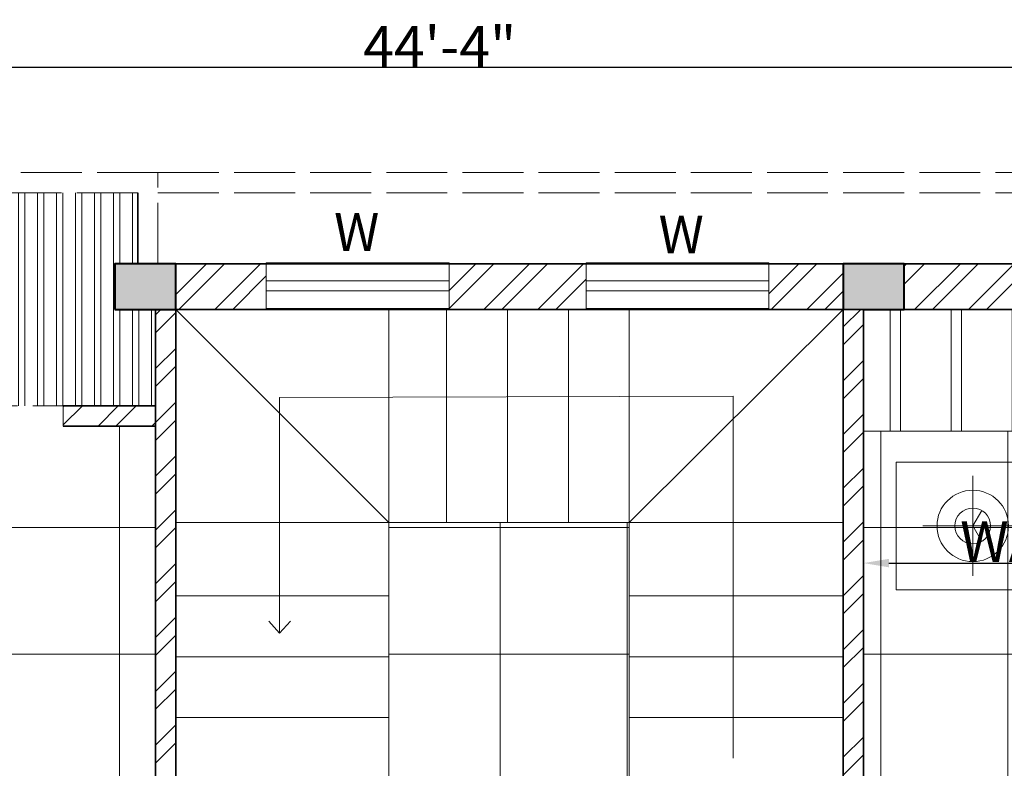
# Model space of a CAD drawing. Units: inches. Extents: x 351 to 1738, y -265 to 286.
# Tile 5 of 38: x 565 to 759, y 138 to 286. Entities that reach past the tile are written whole.
import ezdxf

# ---------------------------------------------------------------- set-up
doc = ezdxf.new("R2010")
doc.units = ezdxf.units.IN
doc.header["$MEASUREMENT"] = 0
doc.linetypes.add('ACAD_ISO02W100', pattern=[15, 12, -3])
for name, color, linetype, lineweight in [('A-ANNO-DIMS', 2, 'Continuous', 18), ('A-ANNO-SYMB', 7, 'Continuous', 18), ('A-COLS', 7, 'Continuous', 40), ('A-COLS-PATT', 6, 'Continuous', 13), ('A-DOOR', 3, 'Continuous', 18), ('A-DOOR-OVHD', 3, 'ACAD_ISO02W100', 13), ('A-FLOR-CASE', 9, 'Continuous', 18), ('A-FLOR-OVHD', 1, 'ACAD_ISO02W100', 18), ('A-FLOR-PATT', 9, 'Continuous', 9), ('A-FLOR-STRS', 7, 'Continuous', 18), ('A-FURN', 18, 'Continuous', 13), ('A-GLAZ', 4, 'Continuous', 18), ('A-WALL', 7, 'Continuous', 35), ('A-WALL-PATT', 152, 'Continuous', 13)]:
    doc.layers.add(name, color=color, linetype=linetype, lineweight=lineweight)
doc.styles.add('Annotative', font='arial.ttf')
doc.styles.get("Standard").update_dxf_attribs({"font": 'arial.ttf'})
doc.dimstyles.get("Standard").update_dxf_attribs({"dimtxt": 8, "dimasz": 5, "dimexe": 0.18, "dimexo": 0.0625, "dimgap": 0.09, "dimtad": 1, "dimtoh": 1, "dimzin": 0, "dimdsep": 46, "dimlunit": 4, "dimtxsty": 'Standard', "dimcen": 0, "dimclre": 256, "dimadec": 0, "dimazin": 0, "dimtfac": 1, "dimtofl": 0, "dimtmove": 0, "dimatfit": 3, "dimfxl": 1, "dimtolj": 1, "dimtzin": 0, "dimlwe": -1, "dimarcsym": 0})

# ---------------------------------------------------------------- blocks, each defined once
blk = doc.blocks.new('*D2')
at = {"layer": 'A-ANNO-DIMS', "color": 0, "transparency": 16777216}
for p, q in [((382.16, 256.03), (382.16, 276.92)), ((914.16, 256.03), (914.16, 276.92))]:
    blk.add_line(p, q, dxfattribs=at)
at = {"layer": 'A-ANNO-DIMS', "color": 0, "lineweight": -2, "transparency": 16777216}
blk.add_line((387.16, 276.74), (909.16, 276.74), dxfattribs=at)
at = {"layer": 'A-ANNO-DIMS', "color": 0, "transparency": 16777216}
for points in [[(387.16, 277.57), (387.16, 275.91), (382.16, 276.74)], [(909.16, 277.57), (909.16, 275.91), (914.16, 276.74)]]:
    blk.add_solid(points, dxfattribs=at)
at = {"layer": 'Defpoints', "color": 0, "transparency": 16777216}
for p in [(914.16, 276.74), (382.16, 255.96), (914.16, 255.96)]:
    blk.add_point(p, dxfattribs=at)
at = {"layer": 'A-ANNO-DIMS', "color": 0, "transparency": 16777216, "insert": (648.16, 280.83), "char_height": 8, "attachment_point": 5}
blk.add_mtext('\\A1;44\'-4"', dxfattribs=at)
blk = doc.blocks.new('BED-DOUBLE-W-NIGHTSTANDS')
for p, q in [((30.18, 128.33), (30.18, 86.91)), ((120.72, 126.39), (30.18, 126.39)), ((15.09, 105.9), (15.09, 125.61)), ((135.81, 105.9), (135.81, 125.61)), ((24.95, 115.76), (5.23, 115.76)), ((125.95, 115.76), (145.67, 115.76)), ((30.18, 104.48), (120.72, 104.48)), ((120.32, 98.22), (66.59, 97.46)), ((120.26, 96.67), (65.46, 95.89)), ((120.18, 91.92), (62.88, 91.69)), ((120.19, 90.37), (62.29, 90.13)), ((121.41, 44.95), (28.44, 44.95)), ((121.55, 43.07), (28.44, 43.07)), ((106.08, 28.24), (44.82, 28.24)), ((36.54, 17.05), (36.2, 18.75)), ((47.08, 17.05), (47.42, 18.75)), ((102.76, 17.05), (102.43, 18.75)), ((113.31, 17.05), (113.64, 18.75))]:
    blk.add_line(p, q)
for points in [[(30.18, 103.18), (0, 103.18), (0, 128.33), (150.9, 128.33), (150.9, 103.18), (120.72, 103.18), (120.72, 128.33)], [(16.85, 112.71), (15.09, 115.76), (16.85, 118.81)], [(134.05, 118.81), (135.81, 115.76), (134.05, 112.71)], [(71.64, 104.48), (63.37, 92.97), (60, 84.12), (59.39, 80.15), (54.5, 81.37), (50.53, 83.2), (43.81, 84.12), (36.16, 84.73), (30.05, 84.12), (28.83, 85.34), (34.33, 91.75), (40.14, 96.03), (51.14, 100), (67.6, 104.48)], [(121.56, 54.36), (129.93, 54.36), (129.93, 0), (19.92, 0), (19.92, 54.36), (28.45, 54.36)], [(28.45, 52.61), (21.67, 52.61), (21.67, 1.75), (128.18, 1.75), (128.18, 52.61), (121.53, 52.61)]]:
    blk.add_lwpolyline(points)
for points in [[(38.85, 124.57, 0.074897), (39.03, 114.71, -0.472817)], [(74.74, 114.16, 0.14099), (75.04, 124.22, 0.235245)], [(81.19, 114.16, -0.14099), (80.89, 124.22, -0.235245)], [(112.05, 124.57, -0.074897), (111.87, 114.71, 0.472817)], [(28.51, 71.52, 0.001242), (28.44, 42.89, -0.127202), (25.42, 28.62)], [(121.36, 46.14, 0.056112), (122.46, 37.83, 0.095341), (124.58, 29.84)]]:
    blk.add_lwpolyline(points, format="xyb")
for centre, radius in [((15.09, 115.76), 7.04), ((135.81, 115.76), 7.04), ((15.09, 115.76), 3.52), ((135.81, 115.76), 3.52), ((45.25, 11.58), 0.384), ((104.59, 11.58), 0.384), ((42.74, 7.53), 0.384), ((107.11, 7.53), 0.384)]:
    blk.add_circle(centre, radius)
for centre, radius, start, end in [((122.02, 1560.65), 1438.48, 266.68521, 267.14978), ((59.52, 69.97), 54.73, 82.2196, 99.497), ((71.08, 97.62), 26.89, 81.5249, 103.96), ((82.96, 117.05), 7.46, 63.3437, 106.1026), ((94.14, 98.17), 26.53, 76.3427, 101.1841), ((28.88, 1560.65), 1438.48, 272.85022, 273.31479), ((58.07, 110.76), 19.45, 155.1316, 191.7583), ((92.83, 110.76), 19.45, 348.2417, 24.8684), ((56.95, 109.12), 18.49, 354.0129, 15.8293), ((98.98, 109.12), 18.49, 164.1707, 185.9871), ((44.23, 126.34), 20.22, 255.1039, 281.0369), ((54.88, 140.71), 35.07, 258.0397, 289.2615), ((69.08, 133.05), 26.61, 259.8617, 283.6238), ((83.97, 114.44), 8, 245.0183, 288.5407), ((97.94, 124.85), 19.21, 243.8761, 286.1746), ((106.67, 126.34), 20.22, 258.9631, 284.8961), ((391.24, 86.04), 271.14, 176.1, 180.9282), ((-109.53, 81.59), 138.41, 355.8294, 1.553), ((31.41, 138.78), 56.95, 267.4519, 281.3392), ((45.02, 70.89), 12.28, 66.2616, 101.3392), ((69.87, 137.17), 58.52, 250.1194, 259.3383), ((473.78, 76.18), 353.69, 179.1145, 184.8735), ((59.05, 80.02), 0.364, 268.8623, 19.7536), ((123.44, 29.07), 1.38, 246.5219, 33.8264), ((26.8, 28.72), 1.39, 183.98, 297.3412), ((43.02, -128.84), 157.09, 89.3433, 95.6887), ((26.22, 17.62), 11.42, 33.6671, 63.2997), ((41.52, 24.41), 5.82, 145.785, 184.7304), ((30.41, 27.13), 6.25, 328.8218, 9.1554), ((38.15, 26.57), 1.82, 120.0293, 142.325), ((35.25, 25.5), 4.81, 289.2822, 29.1751), ((37.38, 26.93), 2.26, 311.5653, 23.8354), ((38.15, 26.57), 1.82, 44.4517, 63.558), ((48.37, 25.5), 4.81, 150.8249, 250.7178), ((46.24, 26.93), 2.26, 156.1646, 228.4347), ((45.47, 26.57), 1.82, 113.229, 135.5483), ((45.47, 26.57), 1.82, 37.675, 66.7144), ((42.1, 24.41), 5.82, 355.2696, 34.215), ((53.21, 27.13), 6.25, 169.7133, 211.1782), ((57.4, 17.62), 11.42, 111.4941, 146.3329), ((92.44, 17.62), 11.42, 33.6671, 68.5059), ((107.75, 24.41), 5.82, 145.785, 184.7304), ((96.63, 27.13), 6.25, 328.8218, 10.2867), ((104.38, 26.57), 1.82, 113.2856, 142.325), ((101.48, 25.5), 4.81, 289.2822, 29.1751), ((104.38, 26.57), 1.82, 44.4517, 66.7144), ((103.61, 26.93), 2.26, 311.5653, 23.8354), ((110.71, -118.52), 146.84, 85.2402, 91.8035), ((114.6, 25.5), 4.81, 150.8249, 250.7178), ((112.47, 26.93), 2.26, 156.1646, 228.4347), ((111.7, 26.57), 1.82, 106.6343, 135.5483), ((111.7, 26.57), 1.82, 37.675, 72.5814), ((108.32, 24.41), 5.82, 355.2696, 34.215), ((119.44, 27.13), 6.25, 169.249, 211.1782), ((123.63, 17.62), 11.42, 113.6453, 146.3329), ((32.87, 23.1), 2.55, 84.4856, 181.0538), ((32.09, 21.21), 4.54, 355.2933, 76.921), ((40.93, 22.93), 3.09, 131.5653, 195.1471), ((34.52, 24.63), 4.34, 7.436, 29.9149), ((42.69, 22.93), 3.09, 344.8529, 48.4347), ((49.1, 24.63), 4.34, 150.0851, 172.564), ((51.53, 21.21), 4.54, 103.079, 184.7067), ((50.75, 23.1), 2.55, 358.9462, 95.5144), ((99.1, 23.1), 2.55, 84.4856, 181.0538), ((98.32, 21.21), 4.54, 355.2933, 76.921), ((107.16, 22.93), 3.09, 131.5653, 195.1471), ((100.75, 24.63), 4.34, 7.436, 29.9149), ((108.92, 22.93), 3.09, 344.8529, 48.4347), ((115.33, 24.63), 4.34, 150.0851, 172.564), ((117.76, 21.21), 4.54, 103.079, 184.7067), ((116.98, 23.1), 2.55, 358.9462, 95.5144), ((34.67, 20.3), 3.75, 299.9085, 73.1337), ((48.95, 20.3), 3.75, 106.8663, 240.0915), ((100.89, 20.3), 3.75, 299.9085, 73.1337), ((115.18, 20.3), 3.75, 106.8663, 240.0915), ((33.91, 22.74), 3.61, 174.9449, 262.8857), ((35.33, 24.1), 3.5, 201.5819, 291.4221), ((37.04, 21.88), 0.937, 257.3041, 15.1471), ((46.58, 21.88), 0.937, 164.8529, 282.6959), ((48.29, 24.1), 3.5, 248.5779, 338.4181), ((49.7, 22.74), 3.61, 277.1143, 5.0551), ((100.14, 22.74), 3.61, 174.9449, 262.8857), ((101.56, 24.1), 3.5, 201.5819, 291.4221), ((103.27, 21.88), 0.937, 257.3041, 15.1471), ((112.81, 21.88), 0.937, 164.8529, 282.6959), ((114.52, 24.1), 3.5, 248.5779, 338.4181), ((115.93, 22.74), 3.61, 277.1143, 5.0551), ((28.59, 21.91), 7.12, 301.2614, 341.7045), ((33.29, 23.54), 4.38, 272.3591, 324.0401), ((28.53, 21.34), 8.1, 326.2883, 356.5076), ((41.52, 24.41), 5.82, 212.7011, 216.3445), ((42.24, 20.46), 0.291, 102.7051, 280.4384), ((42.21, 20.63), 0.473, 280.4384, 100.4136), ((42.1, 24.41), 5.82, 323.6555, 327.2989), ((50.33, 23.54), 4.38, 215.9599, 267.6409), ((55.09, 21.34), 8.1, 183.4924, 213.7117), ((55.02, 21.91), 7.12, 198.2955, 238.7386), ((76.66, 18.28), 1.63, 63.0274, 163.8037), ((75, 22.1), 3.37, 271.4585, 315.3727), ((78.22, 18.28), 1.63, 16.1963, 116.9726), ((79.87, 22.1), 3.37, 224.6273, 268.5415), ((94.82, 21.91), 7.12, 301.2614, 341.7045), ((99.52, 23.54), 4.38, 272.3591, 324.0401), ((94.76, 21.34), 8.1, 326.2883, 356.5076), ((107.75, 24.41), 5.82, 212.7011, 216.3445), ((107.64, 20.63), 0.473, 79.5864, 259.5616), ((107.6, 20.46), 0.291, 259.5616, 77.2949), ((108.32, 24.41), 5.82, 323.6555, 327.2989), ((116.56, 23.54), 4.38, 215.9599, 267.6409), ((121.32, 21.34), 8.1, 183.4924, 213.7117), ((121.25, 21.91), 7.12, 198.2955, 238.7386), ((33.08, 16.92), 2.26, 80.264, 250.8688), ((52.7, 12.86), 12.5, 153.0032, 159.8941), ((40.82, 19.78), 2.42, 285.5129, 293.6099), ((42.4, 17.05), 0.792, 87.3579, 140.4944), ((40.57, 19.33), 2.39, 301.164, 321.5612), ((38.63, 19.74), 4.26, 324.6898, 333.4936), ((50.53, 16.92), 2.26, 289.1312, 99.736), ((76.62, -0.91), 19.71, 94.4623, 172.255), ((76.71, 17.27), 2.19, 137.7873, 219.1145), ((74.23, 17.34), 1.65, 298.5391, 58.3627), ((76.37, 15.9), 3.12, 45.5411, 114.3101), ((79.21, 31.89), 13.79, 252.593, 267.2582), ((76.7, 18.68), 1.61, 177.7585, 283.852), ((79.8, 20.35), 4.98, 198.9159, 238.011), ((78.5, 15.9), 3.12, 65.6899, 134.4589), ((75.66, 31.89), 13.79, 272.7418, 287.407), ((77.04, 17.32), 0.213, 283.852, 219.9245), ((77.82, 17.4), 0.128, 320.1909, 256.0209), ((75.07, 20.35), 4.98, 301.989, 341.0841), ((78.18, 18.68), 1.61, 256.148, 2.2415), ((80.65, 17.34), 1.65, 121.6373, 241.4609), ((78.17, 17.27), 2.19, 320.8855, 42.2127), ((77.62, 3.64), 15.25, 352.8636, 81.8197), ((99.31, 16.92), 2.26, 80.264, 250.8688), ((109.28, 19.33), 2.39, 218.4388, 238.836), ((107.45, 17.05), 0.792, 39.5056, 92.6421), ((111.22, 19.74), 4.26, 206.5064, 215.3102), ((109.03, 19.78), 2.42, 246.3901, 254.4871), ((97.15, 12.86), 12.5, 20.1059, 26.9968), ((116.76, 16.92), 2.26, 289.1312, 99.736), ((32.62, 14.47), 1.39, 63.9755, 143.2681), ((32.54, 17.61), 2.83, 265.969, 344.3045), ((35.59, 13.85), 3.01, 96.1662, 141.5825), ((40.58, 15.96), 0.792, 101.3256, 154.4621), ((39.44, 18.65), 2.39, 280.2588, 300.656), ((39.99, 20.56), 4.26, 268.3264, 277.1302), ((52.7, 12.86), 12.5, 163.5842, 183.8277), ((38.92, 18.64), 2.42, 308.2101, 316.3071), ((40.41, 17.05), 0.724, 278.3432, 4.2869), ((40.01, 17.68), 1.26, 300.656, 332.6341), ((40.96, 16.85), 0.307, 55.7657, 157.4417), ((41.44, 17.14), 0.307, 84.3784, 186.0543), ((41.15, 18.37), 1.26, 269.1859, 301.164), ((41.52, 17.71), 0.724, 237.5332, 323.4768), ((48.03, 13.85), 3.01, 38.4175, 83.8338), ((51.08, 17.61), 2.83, 195.6955, 274.031), ((51, 14.47), 1.39, 36.7319, 116.0245), ((77.29, 16.34), 0.245, 238.011, 71.5592), ((77.33, 16.45), 0.119, 71.5592, 188.0167), ((77.58, 16.34), 0.245, 108.4408, 301.989), ((77.54, 16.45), 0.119, 351.9833, 108.4408), ((98.85, 14.47), 1.39, 63.9755, 143.2681), ((98.77, 17.61), 2.83, 265.969, 344.3045), ((101.82, 13.85), 3.01, 96.1662, 141.5825), ((108.33, 17.71), 0.724, 216.5232, 302.4668), ((108.7, 18.37), 1.26, 238.836, 270.8141), ((108.41, 17.14), 0.307, 353.9457, 95.6216), ((109.44, 17.05), 0.724, 175.7131, 261.6568), ((108.89, 16.85), 0.307, 22.5583, 124.2343), ((109.84, 17.68), 1.26, 207.3659, 239.344), ((97.15, 12.86), 12.5, 356.1723, 16.4158), ((110.93, 18.64), 2.42, 223.6929, 231.7899), ((110.41, 18.65), 2.39, 239.344, 259.7412), ((109.86, 20.56), 4.26, 262.8698, 271.6736), ((109.27, 15.96), 0.792, 25.5379, 78.6744), ((117.31, 17.61), 2.83, 195.6955, 274.031), ((114.26, 13.85), 3.01, 38.4175, 83.8338), ((117.23, 14.47), 1.39, 36.7319, 116.0245), ((31.17, 13.79), 1.63, 92.9516, 193.728), ((27.83, 16.28), 3.37, 301.3827, 345.2969), ((32.11, 11.59), 3.12, 75.4653, 144.2343), ((26.59, 26.86), 13.79, 282.5173, 297.1824), ((38.34, 14.46), 0.641, 101.5637, 142.6358), ((37.8, 13.86), 0.384, 273.2768, 86.7232), ((38.25, 14.23), 0.367, 91.1081, 181.8675), ((38.64, 13.49), 0.794, 80.3487, 133.6538), ((38.5, 14.15), 0.629, 229.7889, 317.6792), ((37.82, 14.96), 0.924, 288.7263, 352.5032), ((37.79, 12.81), 0.893, 355.053, 68.3618), ((38.49, 12.66), 1.26, 83.0852, 105.7171), ((38.45, 14.92), 0.297, 345.2356, 144.9248), ((38.72, 13.95), 0.331, 317.6792, 80.3487), ((51.51, 11.59), 3.12, 35.7657, 104.5347), ((57.03, 26.86), 13.79, 242.8176, 257.4827), ((52.45, 13.79), 1.63, 346.272, 87.0484), ((55.79, 16.28), 3.37, 194.7031, 238.6173), ((97.39, 13.79), 1.63, 92.9516, 193.728), ((94.06, 16.28), 3.37, 301.3827, 345.2969), ((98.34, 11.59), 3.12, 75.4653, 144.2343), ((92.82, 26.86), 13.79, 282.5173, 297.1824), ((111.13, 13.95), 0.331, 99.6513, 222.3208), ((111.35, 14.15), 0.629, 222.3208, 310.2111), ((111.21, 13.49), 0.794, 46.3462, 99.6513), ((111.4, 14.92), 0.297, 35.0752, 194.7644), ((112.03, 14.96), 0.924, 187.4968, 251.2737), ((112.06, 12.81), 0.893, 111.6382, 184.947), ((111.36, 12.66), 1.26, 74.2829, 96.9148), ((111.6, 14.23), 0.367, 358.1325, 88.8919), ((111.51, 14.46), 0.641, 37.3642, 78.4363), ((112.04, 13.86), 0.384, 93.2768, 266.7232), ((117.74, 11.59), 3.12, 35.7657, 104.5347), ((123.26, 26.86), 13.79, 242.8176, 257.4827), ((122.02, 16.28), 3.37, 194.7031, 238.6173), ((118.68, 13.79), 1.63, 346.272, 87.0484), ((7, -0.91), 19.71, 7.745, 41.8856), ((40.71, -2.86), 19.71, 124.3865, 158.5908), ((31.71, 12.94), 2.19, 167.7115, 249.0387), ((29.53, 11.76), 1.65, 328.4633, 88.2869), ((32.86, 17.16), 4.98, 228.8402, 267.9352), ((31.01, 14.16), 1.61, 207.6827, 313.7762), ((31.97, 13.15), 0.213, 313.7762, 249.7183), ((32.66, 12.55), 0.119, 101.4834, 217.9409), ((32.69, 12.42), 0.245, 267.9352, 101.4834), ((38.33, 13.15), 0.634, 217.7621, 259.0403), ((39.01, 14), 1.17, 203.4276, 227.6104), ((38.39, 12.76), 0.295, 232.4737, 355.053), ((29.78, 2.23), 14.33, 43.1541, 52.0459), ((39.68, 10.88), 0.792, 101.3256, 154.4621), ((38.02, 13.56), 2.42, 308.2101, 316.3071), ((39.51, 11.97), 0.724, 278.3432, 4.2869), ((39.11, 12.61), 1.26, 300.656, 332.6341), ((40.06, 11.77), 0.307, 55.7657, 157.4417), ((46.48, 12.55), 6.27, 184.756, 209.2041), ((55.5, 25.89), 20.62, 222.2412, 232.1744), ((43.25, 11.76), 1.06, 272.8499, 356.1226), ((42.31, 12.15), 1.75, 304.5369, 16.3699), ((44.74, 11.66), 1.24, 127.3105, 187.9252), ((43.04, 11.8), 1.27, 355.0106, 41.658), ((44.83, 12.11), 0.524, 126.1046, 271.4281), ((44.77, 12.26), 0.377, 353.7526, 131.7054), ((44.42, 11.81), 0.529, 0.0645, 61.1507), ((44.54, 12.26), 0.604, 311.8413, 355.7877), ((45.79, 12.17), 0.641, 101.5637, 176.365), ((45.7, 11.94), 0.367, 91.1081, 181.8675), ((46.09, 11.2), 0.794, 80.3487, 133.6538), ((45.27, 12.68), 0.924, 288.7263, 352.5032), ((45.9, 12.63), 0.297, 345.2356, 144.9248), ((46.17, 11.66), 0.331, 317.6792, 80.3487), ((47.12, 4.22), 7.52, 87.1071, 94.7585), ((50.93, 12.42), 0.245, 78.5166, 272.0648), ((50.76, 17.16), 4.98, 272.0648, 311.1598), ((50.96, 12.55), 0.119, 322.0591, 78.5166), ((52.61, 14.16), 1.61, 226.2238, 332.3173), ((51.67, 13.23), 0.128, 290.2667, 226.2271), ((54.09, 11.76), 1.65, 91.7131, 211.5367), ((51.9, 12.94), 2.19, 290.9613, 12.2885), ((42.91, -2.86), 19.71, 21.4092, 55.6135), ((106.94, -2.86), 19.71, 124.3865, 158.5908), ((97.94, 12.94), 2.19, 167.7115, 249.0387), ((97.24, 14.16), 1.61, 207.6827, 313.7762), ((99.09, 17.16), 4.98, 228.8402, 267.9352), ((95.76, 11.76), 1.65, 328.4633, 88.2869), ((98.2, 13.15), 0.213, 313.7762, 249.7183), ((98.89, 12.55), 0.119, 101.4834, 217.9409), ((98.92, 12.42), 0.245, 267.9352, 101.4834), ((102.73, 4.22), 7.52, 85.2415, 92.8929), ((103.68, 11.66), 0.331, 99.6513, 222.3208), ((103.76, 11.2), 0.794, 46.3462, 99.6513), ((103.95, 12.63), 0.297, 35.0752, 194.7644), ((104.58, 12.68), 0.924, 187.4968, 251.2737), ((104.15, 11.94), 0.367, 358.1325, 88.8919), ((104.06, 12.17), 0.641, 3.635, 78.4363), ((105.08, 12.26), 0.377, 48.2946, 186.2474), ((105.3, 12.26), 0.604, 184.2123, 228.1587), ((105.43, 11.81), 0.529, 118.8493, 179.9355), ((105.02, 12.11), 0.524, 268.5719, 53.8954), ((106.81, 11.8), 1.27, 138.342, 184.9894), ((106.6, 11.76), 1.06, 183.8774, 267.1501), ((107.53, 12.15), 1.75, 163.6301, 235.4631), ((105.1, 11.66), 1.24, 352.0748, 52.6895), ((94.35, 25.89), 20.62, 307.8256, 317.7588), ((103.37, 12.55), 6.27, 330.7959, 355.244), ((110.34, 11.97), 0.724, 175.7131, 261.6568), ((120.07, 2.23), 14.33, 127.9541, 136.8459), ((109.79, 11.77), 0.307, 22.5583, 124.2343), ((110.74, 12.61), 1.26, 207.3659, 239.344), ((111.83, 13.56), 2.42, 223.6929, 231.7899), ((110.17, 10.88), 0.792, 25.5379, 78.6744), ((111.46, 12.76), 0.295, 184.947, 307.5263), ((110.83, 14), 1.17, 312.3896, 336.5724), ((111.52, 13.15), 0.634, 280.9597, 322.2379), ((117.16, 12.42), 0.245, 78.5166, 272.0648), ((116.99, 17.16), 4.98, 272.0648, 311.1598), ((117.18, 12.55), 0.119, 322.0591, 78.5166), ((118.84, 14.16), 1.61, 226.2238, 332.3173), ((117.9, 13.23), 0.128, 290.2667, 226.2271), ((120.32, 11.76), 1.65, 91.7131, 211.5367), ((118.13, 12.94), 2.19, 290.9613, 12.2885), ((109.14, -2.86), 19.71, 21.4092, 55.6135), ((142.85, -0.91), 19.71, 138.1144, 172.255), ((38.54, 13.57), 2.39, 280.2588, 300.656), ((39.09, 15.48), 4.26, 268.3264, 277.1302), ((39.94, 9.49), 0.429, 146.8636, 236.9021), ((45.99, 18.94), 11.23, 235.1882, 238.8844), ((40.68, 10.11), 1.16, 199.4799, 267.6828), ((47.12, 4.22), 7.52, 120.544, 139.818), ((42.5, 11.35), 1.03, 321.7607, 7.9252), ((42.71, 9.86), 1.03, 8.7227, 54.8872), ((42.77, 9.04), 1.75, 0.278, 72.111), ((43.55, 9.68), 1.06, 20.5253, 88.5375), ((44.96, 10.21), 1.24, 188.7227, 249.3375), ((44.45, 10.86), 0.381, 148.0499, 225.6268), ((47.12, 4.22), 7.52, 113.0501, 113.8477), ((45.15, 10.42), 1.21, 104.7558, 148.0499), ((44.47, 11.29), 0.758, 247.4086, 351.4386), ((43.37, 9.59), 1.27, 334.9899, 21.6373), ((44.68, 11.26), 0.255, 262.906, 7.132), ((45.78, 10.87), 0.634, 151.2196, 259.0403), ((46.46, 11.71), 1.17, 203.4276, 227.6104), ((45.95, 11.86), 0.629, 229.7889, 317.6792), ((45.24, 10.53), 0.893, 355.053, 68.3618), ((45.94, 10.38), 1.26, 83.0852, 105.7171), ((45.84, 10.48), 0.295, 232.4737, 355.053), ((103.9, 11.86), 0.629, 222.3208, 310.2111), ((104.61, 10.53), 0.893, 111.6382, 184.947), ((104.01, 10.48), 0.295, 184.947, 307.5263), ((103.91, 10.38), 1.26, 74.2829, 96.9148), ((103.38, 11.71), 1.17, 312.3896, 336.5724), ((104.07, 10.87), 0.634, 280.9597, 28.7804), ((105.38, 11.29), 0.758, 188.5614, 292.5914), ((105.16, 11.26), 0.255, 172.868, 277.094), ((104.7, 10.42), 1.21, 31.9501, 75.2442), ((106.48, 9.59), 1.27, 158.3627, 205.0101), ((106.3, 9.68), 1.06, 91.4625, 159.4747), ((107.08, 9.04), 1.75, 107.889, 179.722), ((104.89, 10.21), 1.24, 290.6625, 351.2773), ((102.73, 4.22), 7.52, 66.1523, 66.9499), ((105.4, 10.86), 0.381, 314.3732, 31.9501), ((107.13, 9.86), 1.03, 125.1128, 171.2773), ((107.35, 11.35), 1.03, 172.0748, 218.2393), ((102.73, 4.22), 7.52, 40.182, 59.456), ((109.17, 10.11), 1.16, 272.3172, 340.5201), ((103.85, 18.94), 11.23, 301.1156, 304.8118), ((111.31, 13.57), 2.39, 239.344, 259.7412), ((109.9, 9.49), 0.429, 303.0979, 33.1364), ((110.76, 15.48), 4.26, 262.8698, 271.6736), ((40.55, 9.68), 1, 212.8155, 277.3992), ((39.97, 9.01), 1.16, 266.9701, 338.2913), ((33.85, 17.3), 11.23, 302.6784, 306.3746), ((40.26, 8.09), 0.429, 214.3538, 304.3923), ((40.42, 9.71), 0.444, 238.8844, 314.2646), ((40.33, 8.72), 1, 280.3057, 17.1958), ((40.24, 8.61), 0.444, 306.3746, 21.7548), ((40.96, 8.9), 0.335, 19.3605, 201.7548), ((40.97, 9.16), 0.335, 311.8703, 134.2646), ((47.27, 6.1), 6.69, 153.7819, 158.2913), ((41.94, 10.67), 1.75, 247.2305, 319.0635), ((41.36, 10.08), 1.03, 264.4544, 310.6188), ((46.48, 12.55), 6.27, 214.0033, 222.4917), ((42.12, 9.68), 1.06, 218.3208, 298.8162), ((42.32, 8.06), 0.524, 126.1046, 271.4281), ((42.26, 8.21), 0.377, 353.7526, 131.7054), ((42.84, 8.36), 1.24, 70.0041, 130.6188), ((41.9, 7.76), 0.529, 0.0645, 61.1507), ((42.03, 8.21), 0.604, 311.8413, 355.7877), ((42.04, 9.87), 1.27, 297.7043, 344.3516), ((43.27, 8.12), 0.641, 101.5637, 176.365), ((43.19, 7.89), 0.367, 91.1081, 181.8675), ((43.58, 7.15), 0.794, 80.3487, 133.6538), ((42.76, 8.63), 0.924, 288.7263, 352.5032), ((43.39, 8.58), 0.297, 345.2356, 144.9248), ((43.66, 7.61), 0.331, 317.6792, 80.3487), ((75.11, -11.46), 19.71, 94.4623, 117.4146), ((75.2, 6.72), 2.19, 137.7873, 219.1145), ((72.72, 6.78), 1.65, 298.5391, 58.3627), ((75.15, 7.73), 1.63, 63.0274, 163.8037), ((73.5, 11.55), 3.37, 271.4585, 315.3727), ((74.86, 5.35), 3.12, 45.5411, 114.3101), ((78.3, 9.8), 4.98, 198.9159, 238.011), ((77.71, 21.34), 13.79, 252.593, 267.2582), ((75.19, 8.12), 1.61, 177.7585, 283.852), ((80.01, 5.35), 3.12, 65.6899, 134.4589), ((77.17, 21.34), 13.79, 272.7418, 287.407), ((79.73, 7.73), 1.63, 16.1963, 116.9726), ((81.38, 11.55), 3.37, 224.6273, 268.5415), ((76.58, 9.8), 4.98, 301.989, 341.0841), ((79.69, 8.12), 1.61, 256.148, 2.2415), ((82.16, 6.78), 1.65, 121.6373, 241.4609), ((79.68, 6.72), 2.19, 320.8855, 42.2127), ((79.76, -11.46), 19.71, 62.5854, 85.5377), ((106.19, 7.61), 0.331, 99.6513, 222.3208), ((106.27, 7.15), 0.794, 46.3462, 99.6513), ((106.46, 8.58), 0.297, 35.0752, 194.7644), ((107.09, 8.63), 0.924, 187.4968, 251.2737), ((107.01, 8.36), 1.24, 49.3812, 109.9959), ((107.91, 10.67), 1.75, 220.9365, 292.7695), ((107.81, 9.87), 1.27, 195.6484, 242.2957), ((106.66, 7.89), 0.367, 358.1325, 88.8919), ((106.58, 8.12), 0.641, 3.635, 78.4363), ((107.59, 8.21), 0.377, 48.2946, 186.2474), ((107.82, 8.21), 0.604, 184.2123, 228.1587), ((107.73, 9.68), 1.06, 241.1838, 321.6792), ((107.94, 7.76), 0.529, 118.8493, 179.9355), ((107.53, 8.06), 0.524, 268.5719, 53.8954), ((108.49, 10.08), 1.03, 229.3812, 275.5456), ((103.37, 12.55), 6.27, 317.5083, 325.9967), ((109.52, 8.72), 1, 162.8042, 259.6943), ((108.88, 9.16), 0.335, 45.7354, 228.1297), ((108.88, 8.9), 0.335, 338.2452, 160.6395), ((102.58, 6.1), 6.69, 21.7087, 26.2181), ((109.88, 9.01), 1.16, 201.7087, 273.0299), ((109.42, 9.71), 0.444, 225.7354, 301.1156), ((109.61, 8.61), 0.444, 158.2452, 233.6254), ((109.3, 9.68), 1, 262.6008, 327.1845), ((116, 17.3), 11.23, 233.6254, 237.3216), ((109.59, 8.09), 0.429, 235.6077, 325.6462), ((41.93, 6.81), 0.381, 148.0499, 225.6268), ((42.64, 6.37), 1.21, 104.7558, 148.0499), ((41.96, 7.24), 0.758, 247.4086, 351.4386), ((42.17, 7.2), 0.255, 262.906, 7.132), ((43.26, 6.82), 0.634, 151.2196, 259.0403), ((43.95, 7.66), 1.17, 203.4276, 227.6104), ((43.44, 7.81), 0.629, 229.7889, 317.6792), ((42.73, 6.48), 0.893, 355.053, 68.3618), ((43.43, 6.33), 1.26, 83.0852, 105.7171), ((43.32, 6.43), 0.295, 232.4737, 355.053), ((66.74, -3.55), 9.6, 91.272, 146.5383), ((70.19, -5.34), 11.97, 107.8504, 143.6964), ((76.48, -8.7), 17.8, 124.0123, 144.053), ((75.53, 6.76), 0.213, 283.852, 219.9245), ((75.79, 5.78), 0.245, 238.011, 71.5592), ((75.83, 5.9), 0.119, 71.5592, 188.0167), ((79.09, 5.78), 0.245, 108.4408, 301.989), ((79.05, 5.9), 0.119, 351.9833, 108.4408), ((79.33, 6.85), 0.128, 320.1909, 256.0209), ((79.59, 5.04), 8.82, 338.117, 6.6195), ((87.68, 2.58), 3.54, 346.3898, 79.0739), ((85.02, 3.07), 4.47, 342.8609, 41.9049), ((106.41, 7.81), 0.629, 222.3208, 310.2111), ((107.12, 6.48), 0.893, 111.6382, 184.947), ((106.52, 6.43), 0.295, 184.947, 307.5263), ((106.42, 6.33), 1.26, 74.2829, 96.9148), ((105.9, 7.66), 1.17, 312.3896, 336.5724), ((106.58, 6.82), 0.634, 280.9597, 28.7804), ((107.89, 7.24), 0.758, 188.5614, 292.5914), ((107.68, 7.2), 0.255, 172.868, 277.094), ((107.21, 6.37), 1.21, 31.9501, 75.2442), ((107.91, 6.81), 0.381, 314.3732, 31.9501), ((16.88, -3.55), 9.6, 33.4617, 60.1116), ((22.26, -1.32), 8.01, 22.5547, 48.9546), ((0.31, 2.98), 27.26, 357.4081, 3.6519), ((61.36, -1.32), 8.01, 131.0454, 157.4453), ((83.31, 2.98), 27.26, 176.3481, 182.5919), ((66.54, 2.98), 27.26, 357.4081, 3.6519), ((88.49, -1.32), 8.01, 22.5547, 48.9546), ((127.59, -1.32), 8.01, 131.0454, 157.4453), ((149.54, 2.98), 27.26, 176.3481, 182.5919), ((132.97, -3.55), 9.6, 119.8884, 146.5383), ((13.43, -5.34), 11.97, 36.3036, 46.4814), ((69.6, -8.61), 10.84, 73.5431, 107.0202), ((85.27, -8.61), 10.84, 72.9798, 106.4569), ((136.42, -5.34), 11.97, 133.5186, 143.6964), ((73.9, -14.2), 16.02, 94.3787, 95.6357), ((82.34, -25.17), 28.63, 109.7217, 109.9028), ((80.98, -14.2), 16.02, 84.3643, 85.6213), ((72.54, -25.17), 28.63, 70.0972, 70.2783)]:
    blk.add_arc(centre, radius, start, end)
blk = doc.blocks.new('WARDROBE-PANELLED')
for p, q in [((5.27, 24), (5.27, 0)), ((7.27, 24), (7.27, 0)), ((17.27, 24), (17.27, 0)), ((19.27, 24), (19.27, 0)), ((29.27, 24), (29.27, 0)), ((31.27, 24), (31.27, 0)), ((41.27, 24), (41.27, 0)), ((43.27, 24), (43.27, 0)), ((53.27, 24), (53.27, 0)), ((55.27, 24), (55.27, 0)), ((65.27, 24), (65.27, 0)), ((67.27, 24), (67.27, 0)), ((77.27, 24), (77.27, 0)), ((79.27, 24), (79.27, 0)), ((89.27, 24), (89.27, 0)), ((91.27, 24), (91.27, 0)), ((101.27, 24), (101.27, 0)), ((103.27, 24), (103.27, 0)), ((113.27, 24), (113.27, 0)), ((115.27, 24), (115.27, 0)), ((125.27, 24), (125.27, 0)), ((127.27, 24), (127.27, 0)), ((137.27, 24), (137.27, 0)), ((139.27, 24), (139.27, 0)), ((149.27, 24), (149.27, 0)), ((151.27, 24), (151.27, 0)), ((161.27, 24), (161.27, 0)), ((163.27, 24), (163.27, 0)), ((0, 0), (173.5, 0))]:
    blk.add_line(p, q)
blk = doc.blocks.new('COL-9x12')
blk.add_lwpolyline([(0, 12), (0, 0), (9, 0), (9, 12)], close=True)
blk = doc.blocks.new('WIN-36')
for p, q in [((0, 5.5), (36, 5.5)), ((0, 3.5), (36, 3.5))]:
    blk.add_line(p, q)
blk.add_lwpolyline([(0, 9), (36, 9), (36, 0), (0, 0)], close=True)
blk = doc.blocks.new('*D48')
at = {"layer": 'A-ANNO-DIMS', "transparency": 16777216}
for p, q in [((731.66, 204.9), (731.66, 178.76)), ((905.16, 204.9), (905.16, 178.76))]:
    blk.add_line(p, q, dxfattribs=at)
at = {"layer": 'A-ANNO-DIMS', "color": 0, "lineweight": -2, "transparency": 16777216}
blk.add_line((736.66, 178.94), (900.16, 178.94), dxfattribs=at)
at = {"layer": 'A-ANNO-DIMS', "color": 0, "transparency": 16777216}
for points in [[(736.66, 179.77), (736.66, 178.1), (731.66, 178.94)], [(900.16, 179.77), (900.16, 178.1), (905.16, 178.94)]]:
    blk.add_solid(points, dxfattribs=at)
at = {"layer": 'Defpoints', "color": 0, "transparency": 16777216}
for p in [(731.66, 204.96), (905.16, 204.96), (905.16, 178.94)]:
    blk.add_point(p, dxfattribs=at)
at = {"layer": 'A-ANNO-DIMS', "color": 0, "transparency": 16777216, "insert": (818.41, 183.17), "char_height": 8, "attachment_point": 5}
blk.add_mtext('\\A1;WARDROBE 14\'-5 1/2" TYP.', dxfattribs=at)

msp = doc.modelspace()

# ---------------------------------------------------------------- hatches: boundary and pattern name
at = {"layer": 'A-COLS-PATT'}
h = msp.add_hatch(color=256, dxfattribs=at)
h.dxf.hatch_style = 1
h.paths.add_polyline_path([(460.155, 237.963), (451.155, 237.963), (451.155, 228.963), (460.155, 228.963)])
h.paths.add_polyline_path([(463.155, 237.963), (460.155, 237.963), (460.155, 228.963), (463.155, 228.963)])
h.paths.add_polyline_path([(391.155, 255.963), (382.155, 255.963), (382.155, 243.963), (391.155, 243.963)])
h.paths.add_polyline_path([(391.155, 210.963), (382.155, 210.963), (382.155, 198.963), (391.155, 198.963)])
h.paths.add_polyline_path([(391.155, -45.037), (382.155, -45.037), (382.155, -57.037), (391.155, -57.037)])
h.paths.add_polyline_path([(460.155, -45.037), (451.155, -45.037), (451.155, -57.037), (460.155, -57.037)])
h.paths.add_polyline_path([(460.155, -161.037), (451.155, -161.037), (451.155, -164.037), (451.155, -173.037), (460.155, -173.037)])
h.paths.add_polyline_path([(391.155, -161.037), (382.155, -161.037), (382.155, -173.037), (391.155, -173.037)])
h.paths.add_polyline_path([(596, -164.037), (584, -164.037), (584, -173.037), (596, -173.037)])
h.paths.add_polyline_path([(596, -50), (584, -50), (584, -59), (596, -59)])
h.paths.add_polyline_path([(596.155, 73.463), (592.155, 73.463), (592.155, 64.463), (596.155, 64.463)])
h.paths.add_polyline_path([(592.155, 73.463), (584.155, 73.463), (584.155, 64.463), (592.155, 64.463)])
h.paths.add_polyline_path([(596.155, 237.963), (584.155, 237.963), (584.155, 228.963), (596.155, 228.963)])
h.paths.add_polyline_path([(739.655, 237.963), (727.655, 237.963), (727.655, 228.963), (739.655, 228.963)])
h.paths.add_polyline_path([(883.515, 237.963), (871.515, 237.963), (871.515, 228.963), (883.515, 228.963)])
h.paths.add_polyline_path([(883.515, 73.463), (871.515, 73.463), (871.515, 64.463), (883.515, 64.463)])
h.paths.add_polyline_path([(731.655, 73.463), (727.655, 73.463), (727.655, 64.463), (731.655, 64.463)])
h.paths.add_polyline_path([(739.515, 73.463), (731.655, 73.463), (731.655, 64.463), (739.515, 64.463)])
h.paths.add_polyline_path([(883.515, -53.037), (871.515, -53.037), (871.515, -57.037), (883.515, -57.037)])
h.paths.add_polyline_path([(883.515, -48.037), (871.515, -48.037), (871.515, -53.037), (883.515, -53.037)])
h.paths.add_polyline_path([(739.515, -48.037), (727.515, -48.037), (727.515, -56.5), (727.516, -57.037), (739.515, -57.037)])
h.paths.add_polyline_path([(883.515, -164.037), (871.515, -164.037), (871.515, -173.037), (883.515, -173.037)])
at = {"layer": 'A-FLOR-PATT', "transparency": 33554559}
h = msp.add_hatch(dxfattribs=at)
h.set_pattern_fill('ANSI32', color=256, scale=10, angle=45)
h.set_pattern_definition([(90, (460.1553, 209.9627), (-3.75, 0), []), (90, (461.4053, 211.2127), (-3.75, 0), [])])
h.paths.add_polyline_path([(584.155, 237.963), (588.655, 237.963), (588.655, 251.963), (460.155, 251.963), (460.155, 237.963), (463.155, 237.963), (463.155, 228.963), (460.155, 228.963), (460.155, 209.963), (538, 209.963), (574, 209.963), (592.155, 209.963), (592.155, 228.963), (584.155, 228.963)])
h = msp.add_hatch(dxfattribs=at)
h.set_pattern_fill('ANSI37', color=256, scale=200, angle=45)
h.set_pattern_definition([(90, (460.077, -164.037), (-25, 0), []), (180, (460.077, -164.037), (-4e-15, -25), [])])
h.paths.add_polyline_path([(727.516, -57.037), (727.515, -57.037), (727.515, -56.5), (727.5, -45), (727.5, -3.5), (727.501, -2.537), (725.797, -2.537), (725.797, -3.037), (721.988, -3.037), (721.988, -2.537), (717.916, -2.537), (717.916, -3.037), (714.106, -3.037), (714.106, -2.537), (710.487, -2.537), (710.487, -3.037), (706.677, -3.037), (706.677, -2.537), (702.965, -2.537), (702.965, -3.037), (699.155, -3.037), (699.155, -2.537), (694.965, -2.537), (694.965, -3.037), (691.155, -3.037), (691.155, -2.537), (679.655, -2.537), (678.797, -2.537), (677.776, -2.537), (676.723, -2.537), (652.655, -2.537), (651.799, -2.537), (650.778, -2.537), (649.725, -2.537), (625.877, -2.537), (624.879, -2.537), (623.857, -2.537), (622.804, -2.537), (596.155, -2.537), (596.155, -3.537), (460.155, -3.537), (460.155, -81.037), (460.077, -99.07), (460.077, -133.967), (460.155, -152.037), (460.155, -164.037), (485.277, -164.037), (545.277, -164.037), (727.655, -164.037)])
h.paths.add_polyline_path([(584, -59), (584, -50), (596, -50), (596, -59)], flags=16)
h.paths.add_polyline_path([(905.155, 204.963), (731.655, 204.963), (731.655, 73.463), (739.515, 73.463), (739.515, 64.463), (731.655, 64.463), (731.655, -3.5), (727.655, -3.5), (727.655, -3.537), (727.5, -45), (731.655, -45), (731.655, -48.037), (739.515, -48.037), (739.515, -53.037), (754, -53.037), (754, -57.037), (748.655, -57.037), (748.655, -147.037), (815.655, -147.037), (815.655, -138.5), (819.655, -138.5), (819.655, -102.5), (815.655, -102.5), (815.655, -57.037), (790, -57.037), (790, -53.037), (871.515, -53.037), (871.515, -48.037), (883.515, -48.037), (883.515, -53.037), (905.155, -53.037)])
h.paths.add_polyline_path([(871.515, 64.463), (871.515, 73.463), (883.515, 73.463), (883.515, 64.463)], flags=16)
h.paths.add_polyline_path([(727.655, 64.463), (685.515, 64.463), (685.515, 186.963), (638.155, 186.963), (638.155, 88.463), (596.155, 88.463), (596.155, 64.463), (584.155, 64.463), (584.155, 73.463), (592.155, 73.463), (592.155, 205.963), (574, 205.963), (574, 209.963), (538, 209.963), (538, 205.963), (536.5, 205.963), (536.5, 180), (489.5, 180), (489.5, 68.655), (460.155, 68.655), (460.155, 64.463), (536.155, 64.463), (536.155, 48.463), (532.155, 48.463), (532.155, 60.463), (460.155, 60.463), (460.155, 0.463), (532.155, 0.463), (532.155, 12.463), (536.155, 12.463), (536.155, 0.463), (596.155, 0.463), (596.155, -0.537), (622.655, -0.537), (623.655, -0.537), (624.655, -0.537), (625.655, -0.537), (649.655, -0.537), (650.576, -0.537), (651.576, -0.537), (652.576, -0.537), (676.655, -0.537), (677.574, -0.537), (678.574, -0.537), (679.574, -0.537), (691.155, -0.537), (691.155, -0.037), (694.965, -0.037), (694.965, -0.537), (699.155, -0.537), (699.155, -0.037), (702.965, -0.037), (702.965, -0.537), (706.677, -0.537), (706.677, -0.037), (710.487, -0.037), (710.487, -0.537), (714.106, -0.537), (714.106, -0.037), (717.916, -0.037), (717.916, -0.537), (721.988, -0.537), (721.988, -0.037), (725.797, -0.037), (725.797, -0.537), (727.655, -0.537)])
h.paths.add_polyline_path([(485.401, 6.538), (461.783, 6.538), (461.783, 51.327), (485.401, 51.327)], flags=16)
h.paths.add_polyline_path([(483.401, 8.538), (463.783, 8.538), (463.783, 49.327), (483.401, 49.327)], flags=0)
h.paths.add_polyline_path([(476.907, 30.5), (476.907, 29.5), (476.907, 26), (475.907, 26), (475.907, 29.5), (474.449, 29.5), (474.449, 26), (473.449, 26), (470.5, 26), (470.5, 27), (473.449, 27), (473.449, 29.5), (470.5, 29.5), (470.5, 32.758), (471.5, 32.758), (471.5, 30.5), (473.407, 30.5), (473.407, 32.897), (473.407, 33.897), (476.907, 33.897), (476.907, 32.897), (474.407, 32.897), (474.407, 30.5)], flags=0)
at = {"layer": 'A-WALL-PATT'}
h = msp.add_hatch(dxfattribs=at)
h.set_pattern_fill('ANSI32', color=256, scale=20)
h.set_pattern_definition([(45, (382.155, -173.037), (-5.3033, 5.3033), []), (45, (385.691, -173.037), (-5.3033, 5.3033), [])])
h.paths.add_polyline_path([(391.155, -57.037), (382.155, -57.037), (382.155, -81.037), (391.155, -81.037)])
h.paths.add_polyline_path([(391.155, 198.963), (382.155, 198.963), (382.155, -45.037), (391.155, -45.037)])
h.paths.add_polyline_path([(391.155, 243.963), (382.155, 243.963), (382.155, 237.963), (382.155, 210.963), (391.155, 210.963)])
h.paths.add_polyline_path([(460.155, 255.963), (391.155, 255.963), (391.155, 246.963), (451.155, 246.963), (451.155, 237.963), (460.155, 237.963), (460.155, 251.963)])
h.paths.add_polyline_path([(404.155, 207.963), (391.155, 207.963), (391.155, 198.963), (404.155, 198.963)])
h.paths.add_polyline_path([(451.155, 207.963), (440.155, 207.963), (440.155, 198.963), (451.155, 198.963)])
h.paths.add_polyline_path([(460.155, 228.963), (451.155, 228.963), (451.155, 74.963), (460.155, 74.963), (460.155, 97.5)])
h.paths.add_polyline_path([(460.155, 60.463), (532.155, 60.463), (532.155, 48.463), (536.155, 48.463), (536.155, 64.463), (460.155, 64.463), (460.155, 62.963), (451.155, 62.963), (451.155, 46.258), (460.155, 46.258)])
h.paths.add_polyline_path([(460.155, -3.537), (596.155, -3.537), (596.155, 0.463), (536.155, 0.463), (536.155, 12.463), (532.155, 12.463), (532.155, 0.463), (460.155, 0.463), (460.155, 10.258), (451.155, 10.258), (451.155, -45.037), (460.155, -45.037)])
h.paths.add_polyline_path([(460.155, -57.037), (451.155, -57.037), (451.155, -81.037), (460.155, -81.037)])
h.paths.add_polyline_path([(460.155, -152.037), (451.155, -152.037), (451.155, -161.037), (460.155, -161.037)])
h.paths.add_polyline_path([(485.277, -164.037), (460.155, -164.037), (460.155, -164.5), (460.155, -173.037), (485.277, -173.037)])
h.paths.add_polyline_path([(584, -164.037), (545.277, -164.037), (545.277, -173.037), (584, -173.037)])
h.paths.add_polyline_path([(631.58, -164.037), (596, -164.037), (596, -173.037), (631.58, -173.037)])
h.paths.add_polyline_path([(871.515, -164.037), (819.655, -164.037), (819.655, -138.5), (815.655, -138.5), (815.655, -164.037), (691.58, -164.037), (691.58, -173.037), (871.515, -173.037)])
h.paths.add_polyline_path([(731.655, -57.037), (727.516, -57.037), (727.655, -164.037), (731.655, -164.037)])
h.paths.add_polyline_path([(914.155, -138), (905.155, -138), (905.155, -164.037), (883.515, -164.037), (883.515, -173.037), (914.155, -173.037)])
h.paths.add_polyline_path([(914.155, -30.189), (905.155, -30.189), (905.155, -53.037), (883.515, -53.037), (883.515, -57.037), (905.155, -57.037), (905.155, -102), (914.155, -102)])
h.paths.add_polyline_path([(871.515, -53.037), (790, -53.037), (790, -57.037), (815.655, -57.037), (815.655, -102.5), (819.655, -102.5), (819.655, -57.037), (871.515, -57.037)])
h.paths.add_polyline_path([(914.155, 120.993), (905.155, 120.993), (905.155, 29.811), (914.155, 29.811)])
h.paths.add_polyline_path([(731.655, 64.463), (727.655, 64.463), (727.655, -3.5), (731.655, -3.5)])
h.paths.add_polyline_path([(481.5, 209.963), (460.155, 209.963), (460.155, 205.963), (481.5, 205.963)])
h.paths.add_polyline_path([(538, 209.963), (517.5, 209.963), (517.5, 205.963), (538, 205.963)])
h.paths.add_polyline_path([(592.155, 209.963), (574, 209.963), (574, 205.963), (592.155, 205.963)])
h.paths.add_polyline_path([(596.155, 228.963), (592.155, 228.963), (592.155, 73.463), (596.155, 73.463)])
h.paths.add_polyline_path([(614, 237.963), (596.155, 237.963), (596.155, 228.963), (614, 228.963)])
h.paths.add_polyline_path([(677, 237.963), (650, 237.963), (650, 228.963), (677, 228.963)])
h.paths.add_polyline_path([(727.655, 237.963), (713, 237.963), (713, 228.963), (727.655, 228.963)])
h.paths.add_polyline_path([(871.515, 237.963), (739.655, 237.963), (739.655, 228.963), (871.515, 228.963)])
h.paths.add_polyline_path([(731.655, 228.963), (727.655, 228.963), (727.655, 73.463), (731.655, 73.463)])
h.paths.add_polyline_path([(914.155, 237.963), (883.515, 237.963), (883.515, 228.963), (905.155, 228.963), (905.155, 180.993), (914.155, 180.993)])

# ---------------------------------------------------------------- linework, layer by layer
at = {"layer": 'A-ANNO-SYMB'}
for points in [[(706.006, 140.473), (706.006, 211.827), (616.629, 211.614), (616.629, 165.102)], [(614.524, 167.504), (616.629, 165.102), (618.733, 167.504)]]:
    msp.add_lwpolyline(points, dxfattribs=at)
at = {"layer": 'A-COLS'}
msp.add_lwpolyline([(731.655, 228.963), (739.655, 228.963), (739.655, 237.963), (727.655, 237.963), (727.655, 228.963)], dxfattribs=at)
at = {"layer": 'A-DOOR'}
msp.add_line((574, 209.963), (574, 205.963), dxfattribs=at)
at = {"layer": 'A-DOOR-OVHD'}
msp.add_line((538, 209.963), (574, 209.963), dxfattribs=at)
at = {"layer": 'A-FLOR-OVHD'}
for p, q in [((592.655, 255.963), (460.155, 255.963)), ((592.655, 237.963), (592.655, 255.963)), ((592.655, 255.963), (914.155, 255.963)), ((588.655, 251.963), (460.155, 251.963)), ((588.655, 251.963), (460.155, 251.963)), ((588.655, 237.963), (588.655, 251.963)), ((592.655, 251.963), (910.155, 251.963))]:
    msp.add_line(p, q, dxfattribs=at)
at = {"layer": 'A-FLOR-STRS'}
for p, q in [((596.155, 228.963), (638.155, 186.963)), ((638.155, 88.463), (638.155, 228.963)), ((649.515, 186.963), (649.515, 228.963)), ((661.515, 186.963), (661.515, 228.963)), ((673.515, 186.963), (673.515, 228.963)), ((685.515, 64.463), (685.515, 228.963)), ((727.655, 228.963), (685.515, 186.963)), ((727.655, 186.963), (596.155, 186.963)), ((638.155, 172.463), (596.155, 172.463)), ((727.515, 172.463), (685.515, 172.463)), ((638.155, 160.463), (596.155, 160.463)), ((727.515, 160.463), (685.515, 160.463)), ((638.155, 148.463), (596.155, 148.463)), ((727.515, 148.463), (685.515, 148.463))]:
    msp.add_line(p, q, dxfattribs=at)
at = {"layer": 'A-WALL'}
for p, q in [((588.655, 237.963), (588.655, 251.963)), ((914.155, 237.963), (588.655, 237.963)), ((596.155, 237.963), (596.155, 64.463)), ((592.155, 228.963), (592.155, 73.463)), ((596.155, 228.963), (905.155, 228.963)), ((727.655, 228.963), (727.655, -3.537)), ((731.655, 228.963), (731.655, 73.463)), ((574, 209.963), (592.155, 209.963)), ((574, 205.963), (592.155, 205.963))]:
    msp.add_line(p, q, dxfattribs=at)

# ---------------------------------------------------------------- block references
at = {"layer": 'A-COLS', "rotation": 90.00000000000075}
msp.add_blockref('COL-9x12', (596.155, 228.962), dxfattribs=at)
at = {"layer": 'A-FLOR-CASE'}
msp.add_blockref('WARDROBE-PANELLED', (731.655, 204.963), dxfattribs=at)
at = {"layer": 'A-FURN'}
msp.add_blockref('BED-DOUBLE-W-NIGHTSTANDS', (738.083, 70.5), dxfattribs=at)
at = {"layer": 'A-GLAZ'}
for p in [(614, 229.115), (677, 229.115)]:
    msp.add_blockref('WIN-36', p, dxfattribs=at)

# ---------------------------------------------------------------- texts
at = {"layer": 'A-ANNO-SYMB', "style": 'Annotative'}
for p in [(627.354, 240.499), (691.287, 239.986)]:
    msp.add_text('W', height=7.433, dxfattribs=at).set_placement(p)

# ---------------------------------------------------------------- dimensions: what is measured, and where the dimension line sits
at = {"layer": 'A-ANNO-DIMS'}
dim = msp.add_linear_dim(base=(914.155, 276.74), p1=(382.155, 255.963), p2=(914.155, 255.963), dimstyle='Standard', override={"dimclrd": 0, "dimclre": 0, "dimclrt": 0}, dxfattribs=at)
dim.commit()
dim.dimension.update_dxf_attribs({"geometry": '*D2', "text_midpoint": (648.155, 280.83)})
dim = msp.add_linear_dim(base=(905.155, 178.938), p1=(731.655, 204.963), p2=(905.155, 204.963), text='WARDROBE <> TYP.', dimstyle='Standard', override={"dimdec": 1, "dimlfac": 1, "dimrnd": 0, "dimzin": 1, "dimdsep": 46, "dimlunit": 4, "dimfrac": 2}, dxfattribs=at)
dim.commit()
dim.dimension.update_dxf_attribs({"geometry": '*D48', "text_midpoint": (818.405, 183.167)})

doc.saveas('drawing.dxf')
